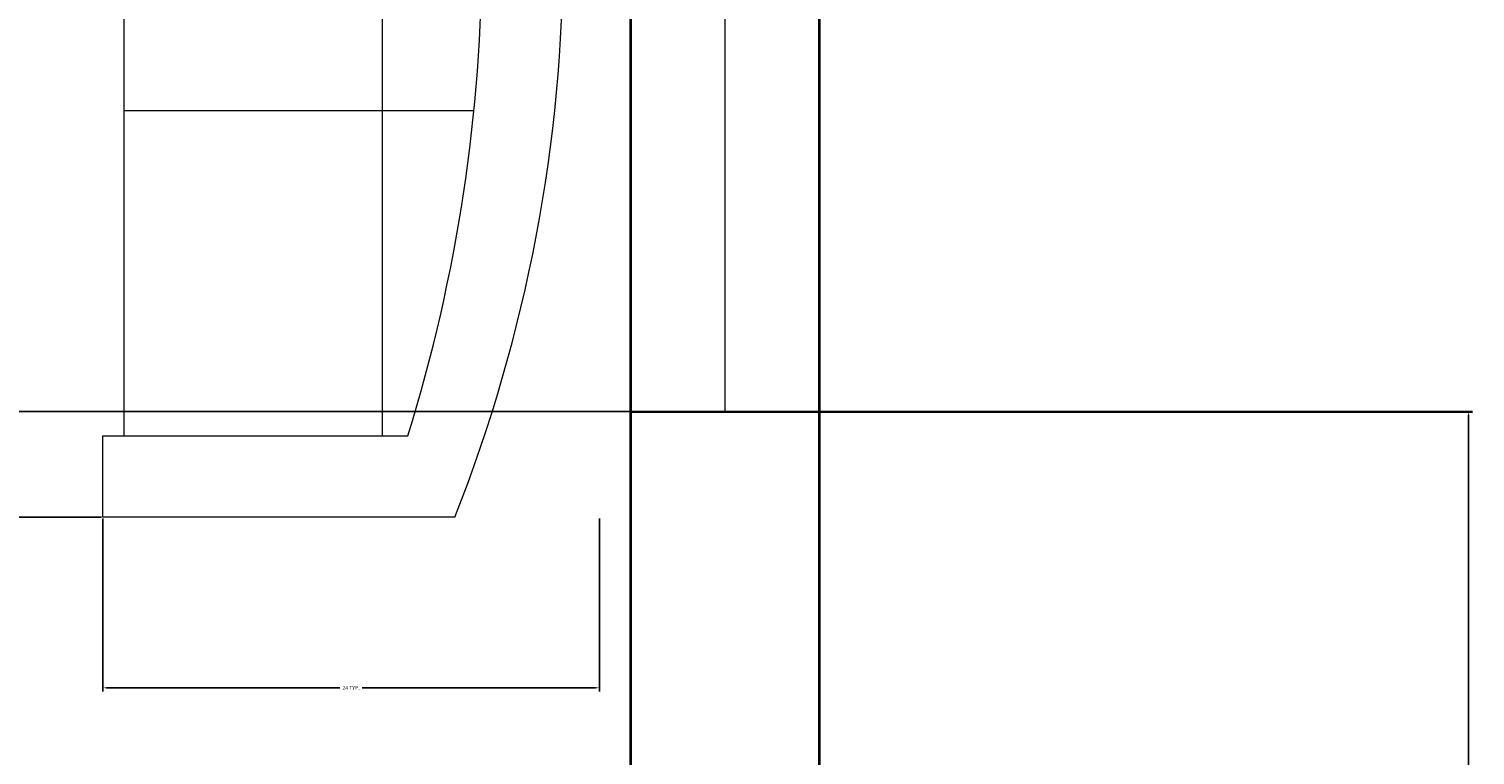
# Model space of a CAD drawing. Units: feet. Extents: x 1654 to 2985, y 1348 to 2230.
# Tile 38 of 53: x 2173 to 2242, y 1785 to 1820. Entities that reach past the tile are written whole.
import ezdxf

# ---------------------------------------------------------------- set-up
doc = ezdxf.new("R2010")
doc.units = ezdxf.units.FT
for name, color, linetype, lineweight in [('A-ANNO-DIMS', 2, 'Continuous', 18), ('A-FURN', 8, 'Continuous', 13), ('A-GLAZ', 4, 'Continuous', 18), ('A-WALL', 7, 'Continuous', 35)]:
    doc.layers.add(name, color=color, linetype=linetype, lineweight=lineweight)
doc.styles.get("Standard").update_dxf_attribs({"font": 'arial.ttf'})
doc.dimstyles.get("Standard").update_dxf_attribs({"dimtxt": 0.18, "dimasz": 0.18, "dimexe": 0.18, "dimexo": 0.0625, "dimgap": 0.09, "dimtad": 0, "dimtih": 1, "dimtoh": 1, "dimdec": 4, "dimzin": 0, "dimdsep": 46, "dimtxsty": 'Standard', "dimcen": 0.09, "dimadec": 0, "dimazin": 0, "dimtfac": 1, "dimtdec": 4, "dimtofl": 0, "dimtmove": 0, "dimatfit": 3, "dimfxl": 1, "dimtolj": 1, "dimtzin": 0, "dimarcsym": 0})

# ---------------------------------------------------------------- blocks, each defined once
blk = doc.blocks.new('Sofa - Roundback 7 ft.')
for p, q in [((11.99997, -32.4421), (11.99998, -6.5971)), ((35.99998, -34), (35.99998, -11.4696)), ((-35.999844, -13.3819), (35.9998, -13.3819)), ((-36.000027, -32.4421), (35.99998, -32.4421))]:
    blk.add_line(p, q)
blk.add_lwpolyline([(41.99998, -8), (41.99998, -34), (35.99998, -34)])
for centre, radius, start, end in [((0, -114.25), 114.25, 68.43141, 111.5686), ((-0.00001, -127.1968), 121.1968, 72.72033, 107.2797)]:
    blk.add_arc(centre, radius, start, end)
blk = doc.blocks.new('WIN-LIVING-EAST')
for p, q in [((4.5, 47.934), (4.5, 0)), ((0, 0), (9, 0))]:
    blk.add_line(p, q)
blk = doc.blocks.new('*D38')
at = {"layer": 'A-ANNO-DIMS', "color": 0, "lineweight": -2, "transparency": 16777216}
for p, q in [((2176.839, 1850.733), (2168.575, 1850.733)), ((2168.755, 1850.553), (2168.755, 1823.764)), ((2168.755, 1796.609), (2168.755, 1823.398)), ((2176.839, 1796.429), (2168.575, 1796.429))]:
    blk.add_line(p, q, dxfattribs=at)
at = {"layer": 'A-ANNO-DIMS', "color": 0, "transparency": 16777216}
for points in [[(2168.725, 1850.553), (2168.785, 1850.553), (2168.755, 1850.733)], [(2168.725, 1796.609), (2168.785, 1796.609), (2168.755, 1796.429)]]:
    blk.add_solid(points, dxfattribs=at)
at = {"layer": 'Defpoints', "color": 0, "transparency": 16777216}
for p in [(2176.901, 1850.733), (2168.755, 1796.429), (2176.901, 1796.429)]:
    blk.add_point(p, dxfattribs=at)
at = {"layer": 'A-ANNO-DIMS', "color": 0, "transparency": 16777216, "insert": (2168.755, 1823.581), "char_height": 0.18, "attachment_point": 5}
blk.add_mtext('\\A1;SOFA 54 TYP.', dxfattribs=at)
blk = doc.blocks.new('*D39')
at = {"layer": 'A-ANNO-DIMS', "color": 0, "lineweight": -2, "transparency": 16777216}
for p, q in [((2176.901, 1796.366), (2176.901, 1788.103)), ((2200.606, 1796.366), (2200.606, 1788.103)), ((2177.081, 1788.283), (2188.224, 1788.283)), ((2200.426, 1788.283), (2189.283, 1788.283))]:
    blk.add_line(p, q, dxfattribs=at)
at = {"layer": 'A-ANNO-DIMS', "color": 0, "transparency": 16777216}
for points in [[(2177.081, 1788.313), (2177.081, 1788.253), (2176.901, 1788.283)], [(2200.426, 1788.313), (2200.426, 1788.253), (2200.606, 1788.283)]]:
    blk.add_solid(points, dxfattribs=at)
at = {"layer": 'Defpoints', "color": 0, "transparency": 16777216}
for p in [(2176.901, 1796.429), (2200.606, 1796.429), (2200.606, 1788.283)]:
    blk.add_point(p, dxfattribs=at)
at = {"layer": 'A-ANNO-DIMS', "color": 0, "transparency": 16777216, "insert": (2188.753, 1788.283), "char_height": 0.18, "attachment_point": 5}
blk.add_mtext('\\A1;24 TYP.', dxfattribs=at)
blk = doc.blocks.new('*D80')
at = {"layer": 'A-ANNO-DIMS', "color": 0, "lineweight": -2, "transparency": 16777216}
for p, q in [((2070.092, 2039.192), (2070.092, 1534.075)), ((2202.092, 2039.192), (2202.092, 1534.075)), ((2070.272, 1534.255), (2135.813, 1534.255)), ((2201.912, 1534.255), (2136.372, 1534.255))]:
    blk.add_line(p, q, dxfattribs=at)
at = {"layer": 'A-ANNO-DIMS', "color": 0, "transparency": 16777216}
for points in [[(2070.272, 1534.285), (2070.272, 1534.225), (2070.092, 1534.255)], [(2201.912, 1534.285), (2201.912, 1534.225), (2202.092, 1534.255)]]:
    blk.add_solid(points, dxfattribs=at)
at = {"layer": 'Defpoints', "color": 0, "transparency": 16777216}
for p in [(2070.092, 2039.255), (2202.092, 2039.255), (2202.092, 1534.255)]:
    blk.add_point(p, dxfattribs=at)
at = {"layer": 'A-ANNO-DIMS', "color": 0, "transparency": 16777216, "insert": (2136.092, 1534.255), "char_height": 0.18, "attachment_point": 5}
blk.add_mtext('\\A1;132', dxfattribs=at)
blk = doc.blocks.new('*D91')
at = {"layer": 'A-ANNO-DIMS', "color": 0, "lineweight": -2, "transparency": 16777216}
for p, q in [((1852.155, 1801.468), (2242.272, 1801.468)), ((2242.092, 1801.288), (2242.092, 1776.544)), ((2242.092, 1751.435), (2242.092, 1776.18)), ((1852.155, 1751.255), (2242.272, 1751.255))]:
    blk.add_line(p, q, dxfattribs=at)
at = {"layer": 'A-ANNO-DIMS', "color": 0, "transparency": 16777216}
for points in [[(2242.062, 1801.288), (2242.122, 1801.288), (2242.092, 1801.468)], [(2242.062, 1751.435), (2242.122, 1751.435), (2242.092, 1751.255)]]:
    blk.add_solid(points, dxfattribs=at)
at = {"layer": 'Defpoints', "color": 0, "transparency": 16777216}
for p in [(1852.092, 1801.468), (2242.092, 1801.468), (1852.092, 1751.255)]:
    blk.add_point(p, dxfattribs=at)
at = {"layer": 'A-ANNO-DIMS', "color": 0, "transparency": 16777216, "insert": (2242.092, 1776.362), "char_height": 0.18, "attachment_point": 5}
blk.add_mtext('\\A1;50.21', dxfattribs=at)
blk = doc.blocks.new('*D96')
at = {"layer": 'A-ANNO-DIMS', "color": 0, "lineweight": -2, "transparency": 16777216}
for p, q in [((2202.155, 1801.437), (2242.272, 1801.437)), ((2242.092, 1801.257), (2242.092, 1776.528)), ((2242.092, 1751.435), (2242.092, 1776.164)), ((2202.155, 1751.255), (2242.272, 1751.255))]:
    blk.add_line(p, q, dxfattribs=at)
at = {"layer": 'A-ANNO-DIMS', "color": 0, "transparency": 16777216}
for points in [[(2242.062, 1801.257), (2242.122, 1801.257), (2242.092, 1801.437)], [(2242.062, 1751.435), (2242.122, 1751.435), (2242.092, 1751.255)]]:
    blk.add_solid(points, dxfattribs=at)
at = {"layer": 'Defpoints', "color": 0, "transparency": 16777216}
for p in [(2202.092, 1801.437), (2242.092, 1801.437), (2202.092, 1751.255)]:
    blk.add_point(p, dxfattribs=at)
at = {"layer": 'A-ANNO-DIMS', "color": 0, "transparency": 16777216, "insert": (2242.092, 1776.346), "char_height": 0.18, "attachment_point": 5}
blk.add_mtext('\\A1;50.18', dxfattribs=at)

msp = doc.modelspace()

# ---------------------------------------------------------------- linework, layer by layer
at = {"layer": 'A-WALL'}
for p, q in [((2211.0924, 2117.2549), (2211.0924, 1742.2549)), ((2202.0924, 1886.2549), (2202.0924, 1751.2549)), ((2211.0924, 1886.2549), (2211.0924, 1565.2549))]:
    msp.add_line(p, q, dxfattribs=at)

# ---------------------------------------------------------------- block references
at = {"layer": 'A-FURN', "xscale": 0.6464854603293951, "yscale": 0.6464854603293951, "zscale": 0.6464854603293951, "rotation": 270}
msp.add_blockref('Sofa - Roundback 7 ft.', (2198.8816, 1823.581), dxfattribs=at)
at = {"layer": 'A-GLAZ'}
msp.add_blockref('WIN-LIVING-EAST', (2202.092, 1801.437), dxfattribs=at)

# ---------------------------------------------------------------- dimensions: what is measured, and where the dimension line sits
at = {"layer": 'A-ANNO-DIMS'}
dim = msp.add_linear_dim(base=(2202.0924, 1534.2549), p1=(2070.0924, 2039.2549), p2=(2202.0924, 2039.2549), dimstyle='Standard', override={"dimdec": 0, "dimlfac": 1, "dimrnd": 0, "dimzin": 0, "dimdsep": 46, "dimlunit": 2}, dxfattribs=at)
dim.commit()
dim.dimension.update_dxf_attribs({"geometry": '*D80', "text_midpoint": (2136.0924, 1534.2549)})
dim = msp.add_linear_dim(base=(2168.7554, 1796.4287), p1=(2176.9011, 1850.7334), p2=(2176.9011, 1796.4287), angle=270, text='SOFA <> TYP.', dimstyle='Standard', override={"dimdec": 0, "dimlfac": 1, "dimrnd": 0, "dimzin": 0, "dimdsep": 46, "dimlunit": 2}, dxfattribs=at)
dim.commit()
dim.dimension.update_dxf_attribs({"geometry": '*D38', "text_midpoint": (2168.7554, 1823.5811)})
for base, p1, p2, picture, middle in [((2242.0924, 1801.4683), (1852.0924, 1751.2549), (1852.0924, 1801.4683), '*D91', (2242.0924, 1776.3616)), ((2242.0924, 1801.4371), (2202.0924, 1751.2549), (2202.0924, 1801.4371), '*D96', (2242.0924, 1776.346))]:
    dim = msp.add_linear_dim(base=base, p1=p1, p2=p2, angle=90, dimstyle='Standard', override={"dimdec": 2, "dimlfac": 1, "dimrnd": 0, "dimzin": 0, "dimdsep": 46, "dimlunit": 2}, dxfattribs=at)
    dim.commit()
    dim.dimension.update_dxf_attribs({"geometry": picture, "text_midpoint": middle})
dim = msp.add_linear_dim(base=(2200.6055, 1788.2829), p1=(2176.9011, 1796.4287), p2=(2200.6055, 1796.4287), text='<> TYP.', dimstyle='Standard', override={"dimdec": 0, "dimlfac": 1, "dimrnd": 0, "dimzin": 0, "dimdsep": 46, "dimlunit": 2}, dxfattribs=at)
dim.commit()
dim.dimension.update_dxf_attribs({"geometry": '*D39', "text_midpoint": (2188.7533, 1788.2829)})

doc.saveas('drawing.dxf')
